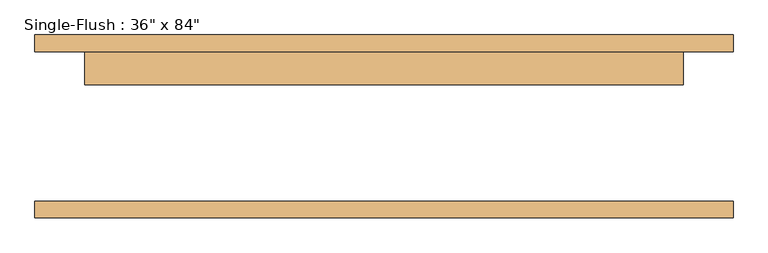
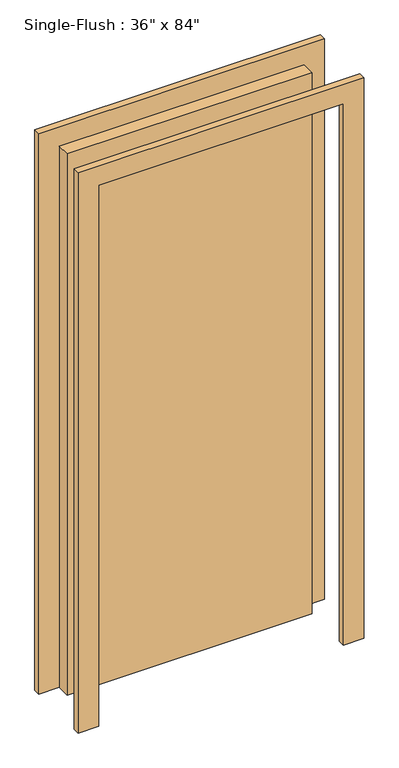
"""IFC4 building model written with IfcOpenShell, lengths in millimetres: door geometry."""

from ifc_helpers import new_model, si_unit, frame, origin, origin_with_axes, place, context, project, spatial, polyline, outline, extrude, source, transform, mapped, element, save


def door_0ca8825f(model_context):
    return source(origin(), model_context, "Body", "SweptSolid", [
        extrude(outline(polyline([(2209.8, -533.4), (0.0, -533.4), (0.0, -457.2), (2133.6, -457.2), (2133.6, 457.2), (0.0, 457.2), (0.0, 533.4), (2209.8, 533.4), (2209.8, -533.4)])), frame((0.0, 114.3, 0.0), z_axis=(0.0, 1.0, 0.0), x_axis=(0.0, 0.0, 1.0)), (0.0, 0.0, 1.0), 25.4),
        extrude(outline(polyline([(2209.8, 533.4), (2209.8, -533.4), (0.0, -533.4), (0.0, -457.2), (2133.6, -457.2), (2133.6, 457.2), (0.0, 457.2), (0.0, 533.4), (2209.8, 533.4)])), frame((0.0, -139.7, 0.0), z_axis=(0.0, 1.0, 0.0), x_axis=(0.0, 0.0, 1.0)), (0.0, 0.0, 1.0), 25.4),
        extrude(outline(polyline([(457.2, 63.5), (-457.2, 63.5), (-457.2, 114.3), (457.2, 114.3), (457.2, 63.5)])), origin_with_axes(), (0.0, 0.0, 1.0), 2133.6),
    ])


if __name__ == "__main__":
    model = new_model("IFC4")
    model_context = context("Model", 3, world=origin())
    ifc_project = project(units=[si_unit("LENGTHUNIT", "METRE", prefix="MILLI")], contexts=[model_context])
    site = spatial("IfcSite", under=ifc_project)
    building = spatial("IfcBuilding", under=site)
    placement = place(None, origin())
    door_shape = door_0ca8825f(model_context)
    element("IfcDoor", 1, ObjectType="Single-Flush : 36\" x 84\"", at=placement, inside=building, context=model_context, shape_type="MappedRepresentation", body=[
        mapped(door_shape, transform((0.0, 0.0, 0.0), x_axis=(1.0, 0.0, 0.0), y_axis=(0.0, 1.0, 0.0), z_axis=(0.0, 0.0, 1.0))),
    ])
    save(model, "model.ifc")

# Revit data of these elements
# Type "Single-Flush : 36\" x 84\""
#   Type Mark = "1"
#   Construction Type Id = "MDOOR"
#   Assembly Code = "C1020"
#   Analytic Construction = "Metal"
#   Thickness = 0' - 2"
#   Heat Transfer Coefficient (U) = 0.651978 BTU/(h·ft²·°F)
#   Height = 7' - 0"
#   Trim Projection Ext = 0' - 1"
#   Trim Projection Int = 0' - 1"
#   Trim Width = 0' - 3"
#   Width = 3' - 0"
#   Define Thermal Properties by = 1
#   Door Material = Door - Panel
#   Frame Material = Door - Frame
#   Visual Light Transmittance = 0
#   Solar Heat Gain Coefficient = 0
#   Function = (empty or 0)
#   Wall Closure = (empty or 0)
# Element 1 (IfcDoor, "Single-Flush : 36\" x 84\"")
#   Materials on its faces: "Door - Frame", "Door - Panel"
# Materials
#   "Door - Panel": class "Wood", colour RGB 210 159 95, transparency 0
#   "Door - Frame": colour RGB 118 70 51, transparency 0
